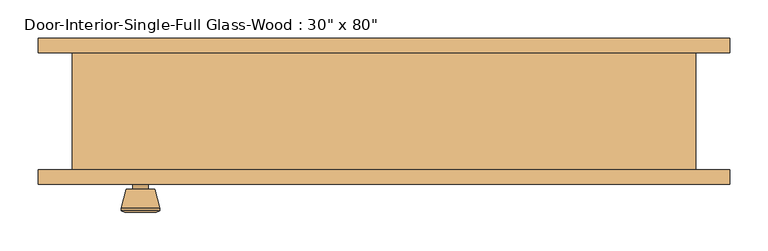
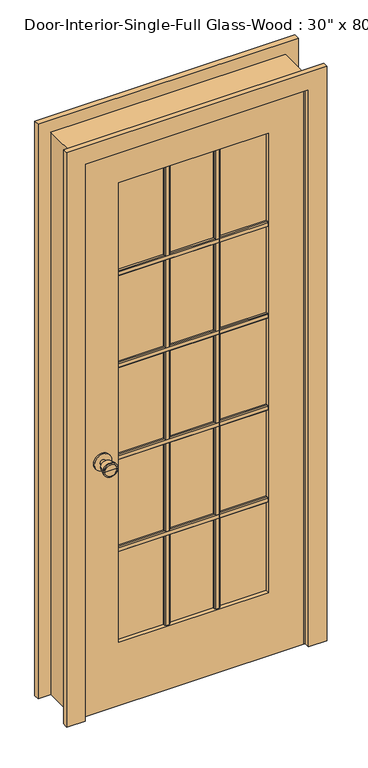
"""IFC4 building model written with IfcOpenShell, lengths in millimetres: door geometry."""

from ifc_helpers import new_model, si_unit, point, frame, frame_2d, origin, place, context, project, spatial, polyline, circle_curve, trimmed, segment, composite_curve, outline, extrude, faceted_brep, source, transform, mapped, element, save
from ifc_brep_helpers import plane_surface, cylinder_surface, revolved_surface, advanced_brep


def door_a0b5ff2a(model_context):
    return source(origin(), model_context, "Body", "SolidModel", [
        extrude(outline(polyline([(-59.055, 1586.23), (-59.055, 1567.18), (-65.405, 1567.18), (-68.58, 1570.355), (-68.58, 1583.055), (-65.405, 1586.23), (-59.055, 1586.23)])), frame((-260.35, 0.0, 0.0), z_axis=(1.0, 0.0, 0.0), x_axis=(0.0, 1.0, 0.0)), (0.0, 0.0, 1.0), 520.7),
        extrude(outline(polyline([(-59.055, 1249.9975), (-59.055, 1230.9475), (-65.405, 1230.9475), (-68.58, 1234.1225), (-68.58, 1246.8225), (-65.405, 1249.9975), (-59.055, 1249.9975)])), frame((-260.35, 0.0, 0.0), z_axis=(1.0, 0.0, 0.0), x_axis=(0.0, 1.0, 0.0)), (0.0, 0.0, 1.0), 520.7),
        extrude(outline(polyline([(-59.055, 913.765), (-59.055, 894.715), (-65.405, 894.715), (-68.58, 897.89), (-68.58, 910.59), (-65.405, 913.765), (-59.055, 913.765)])), frame((-260.35, 0.0, 0.0), z_axis=(1.0, 0.0, 0.0), x_axis=(0.0, 1.0, 0.0)), (0.0, 0.0, 1.0), 520.7),
        extrude(outline(polyline([(-59.055, 577.5325), (-59.055, 558.4825), (-65.405, 558.4825), (-68.58, 561.6575), (-68.58, 574.3575), (-65.405, 577.5325), (-59.055, 577.5325)])), frame((-260.35, 0.0, 0.0), z_axis=(1.0, 0.0, 0.0), x_axis=(0.0, 1.0, 0.0)), (0.0, 0.0, 1.0), 520.7),
        extrude(outline(polyline([(77.2583333, -59.055), (96.3083333, -59.055), (96.3083333, -65.405), (93.1333333, -68.58), (80.4333333, -68.58), (77.2583333, -65.405), (77.2583333, -59.055)])), frame((0.0, 0.0, 231.775), z_axis=(0.0, 0.0, 1.0), x_axis=(1.0, 0.0, 0.0)), (0.0, 0.0, 1.0), 1681.1625),
        extrude(outline(polyline([(-96.3083333, -59.055), (-77.2583333, -59.055), (-77.2583333, -65.405), (-80.4333333, -68.58), (-93.1333333, -68.58), (-96.3083333, -65.405), (-96.3083333, -59.055)])), frame((0.0, 0.0, 231.775), z_axis=(0.0, 0.0, 1.0), x_axis=(1.0, 0.0, 0.0)), (0.0, 0.0, 1.0), 1681.1625),
        extrude(outline(polyline([(-52.07, 1586.23), (-45.72, 1586.23), (-42.545, 1583.055), (-42.545, 1570.355), (-45.72, 1567.18), (-52.07, 1567.18), (-52.07, 1586.23)])), frame((-260.35, 0.0, 0.0), z_axis=(1.0, 0.0, 0.0), x_axis=(0.0, 1.0, 0.0)), (0.0, 0.0, 1.0), 520.7),
        extrude(outline(polyline([(-52.07, 1249.9975), (-45.72, 1249.9975), (-42.545, 1246.8225), (-42.545, 1234.1225), (-45.72, 1230.9475), (-52.07, 1230.9475), (-52.07, 1249.9975)])), frame((-260.35, 0.0, 0.0), z_axis=(1.0, 0.0, 0.0), x_axis=(0.0, 1.0, 0.0)), (0.0, 0.0, 1.0), 520.7),
        extrude(outline(polyline([(-52.07, 913.765), (-45.72, 913.765), (-42.545, 910.59), (-42.545, 897.89), (-45.72, 894.715), (-52.07, 894.715), (-52.07, 913.765)])), frame((-260.35, 0.0, 0.0), z_axis=(1.0, 0.0, 0.0), x_axis=(0.0, 1.0, 0.0)), (0.0, 0.0, 1.0), 520.7),
        extrude(outline(polyline([(-52.07, 577.5325), (-45.72, 577.5325), (-42.545, 574.3575), (-42.545, 561.6575), (-45.72, 558.4825), (-52.07, 558.4825), (-52.07, 577.5325)])), frame((-260.35, 0.0, 0.0), z_axis=(1.0, 0.0, 0.0), x_axis=(0.0, 1.0, 0.0)), (0.0, 0.0, 1.0), 520.7),
        extrude(outline(polyline([(77.2583333, -52.07), (77.2583333, -45.72), (80.4333333, -42.545), (93.1333333, -42.545), (96.3083333, -45.72), (96.3083333, -52.07), (77.2583333, -52.07)])), frame((0.0, 0.0, 231.775), z_axis=(0.0, 0.0, 1.0), x_axis=(1.0, 0.0, 0.0)), (0.0, 0.0, 1.0), 1681.1625),
        extrude(outline(polyline([(-96.3083333, -52.07), (-96.3083333, -45.72), (-93.1333333, -42.545), (-80.4333333, -42.545), (-77.2583333, -45.72), (-77.2583333, -52.07), (-96.3083333, -52.07)])), frame((0.0, 0.0, 231.775), z_axis=(0.0, 0.0, 1.0), x_axis=(1.0, 0.0, 0.0)), (0.0, 0.0, 1.0), 1681.1625),
        advanced_brep(
        [(-317.5, -32.1, 914.4), (-327.5, -32.1, 914.4), (-307.5, -32.1, 914.4), (-297.0241324, 16.9, 914.4), (-337.9758676, 16.9, 914.4), (-317.5, 16.9, 914.4), (-292.5, 15.0721319, 914.4), (-342.5, 15.0721319, 914.4), (-292.5, 11.6084537, 914.4), (-342.5, 11.6084537, 914.4), (-298.863764, -13.1, 914.4), (-336.136236, -13.1, 914.4), (-307.5, -13.1, 914.4), (-327.5, -13.1, 914.4)],
        [
            (0, 1),
            (1, 2, circle_curve(frame((-317.5, -32.1, 914.4), z_axis=(0.0, -1.0, 0.0), x_axis=(-1.0, 0.0, 0.0)), 10.0)),
            (2, 0),
            (2, 1, circle_curve(frame((-317.5, -32.1, 914.4), z_axis=(0.0, -1.0, 0.0), x_axis=(-1.0, 0.0, 0.0)), 10.0)),
            (3, 4, circle_curve(frame((-317.5, 16.9, 914.4), z_axis=(0.0, 1.0, 0.0), x_axis=(-1.0, 0.0, 0.0)), 20.4758676)),
            (4, 5),
            (5, 3),
            (4, 3, circle_curve(frame((-317.5, 16.9, 914.4), z_axis=(0.0, 1.0, 0.0), x_axis=(-1.0, 0.0, 0.0)), 20.4758676)),
            (6, 7, circle_curve(frame((-317.5, 15.0721319, 914.4), z_axis=(0.0, 1.0, 0.0), x_axis=(-1.0, 0.0, 0.0)), 25.0)),
            (7, 4),
            (3, 6),
            (7, 6, circle_curve(frame((-317.5, 15.0721319, 914.4), z_axis=(0.0, 1.0, 0.0), x_axis=(-1.0, 0.0, 0.0)), 25.0)),
            (8, 9, circle_curve(frame((-317.5, 11.6084537, 914.4), z_axis=(0.0, 1.0, 0.0), x_axis=(-1.0, 0.0, 0.0)), 25.0)),
            (9, 7),
            (6, 8),
            (9, 8, circle_curve(frame((-317.5, 11.6084537, 914.4), z_axis=(0.0, 1.0, 0.0), x_axis=(-1.0, 0.0, 0.0)), 25.0)),
            (10, 11, circle_curve(frame((-317.5, -13.1, 914.4), z_axis=(0.0, 1.0, 0.0), x_axis=(-1.0, 0.0, 0.0)), 18.636236)),
            (11, 9),
            (8, 10),
            (11, 10, circle_curve(frame((-317.5, -13.1, 914.4), z_axis=(0.0, 1.0, 0.0), x_axis=(-1.0, 0.0, 0.0)), 18.636236)),
            (12, 13, circle_curve(frame((-317.5, -13.1, 914.4), z_axis=(0.0, 1.0, 0.0), x_axis=(-1.0, 0.0, 0.0)), 10.0)),
            (13, 11),
            (10, 12),
            (13, 12, circle_curve(frame((-317.5, -13.1, 914.4), z_axis=(0.0, 1.0, 0.0), x_axis=(-1.0, 0.0, 0.0)), 10.0)),
            (1, 13),
            (12, 2),
        ],
        [
            plane_surface(frame((-317.5, -32.1, 914.4), z_axis=(0.0, -1.0, 0.0), x_axis=(-1.0, 0.0, 0.0))),
            plane_surface(frame((-317.5, 16.9, 914.4), z_axis=(0.0, 1.0, 0.0), x_axis=(-1.0, 0.0, 0.0))),
            revolved_surface(polyline([(-337.9758676, 16.9, 914.4), (-342.5, 15.0721319, 914.4)]), (-317.5, -32.1, 914.4), (0.0, -1.0, 0.0)),
            cylinder_surface(frame((-317.5, -32.1, 914.4), z_axis=(0.0, -1.0, 0.0), x_axis=(-1.0, 0.0, 0.0)), 25.0),
            revolved_surface(polyline([(-342.5, 11.6084537, 914.4), (-336.136236, -13.1, 914.4)]), (-317.5, -32.1, 914.4), (0.0, -1.0, 0.0)),
            plane_surface(frame((-317.5, -13.1, 914.4), z_axis=(0.0, -1.0, 0.0), x_axis=(-1.0, 0.0, 0.0))),
            cylinder_surface(frame((-317.5, -32.1, 914.4), z_axis=(0.0, -1.0, 0.0), x_axis=(-1.0, 0.0, 0.0)), 10.0),
        ],
        [
            (0, [[1, 2, 3]]),
            (0, [[-3, 4, -1]]),
            (1, [[5, 6, 7]]),
            (1, [[8, -7, -6]]),
            (2, [[9, 10, -5, 11]]),
            (2, [[12, -11, -8, -10]]),
            (3, [[13, 14, -9, 15]]),
            (3, [[16, -15, -12, -14]]),
            (4, [[17, 18, -13, 19]]),
            (4, [[20, -19, -16, -18]]),
            (5, [[21, 22, -17, 23]]),
            (5, [[24, -23, -20, -22]]),
            (6, [[-2, 25, -21, 26]]),
            (6, [[-4, -26, -24, -25]]),
        ],
    ),
        extrude(outline(composite_curve([segment(trimmed(circle_curve(frame_2d((914.4, -317.5)), 30.0), [point((914.4, -347.5))], [point((914.4, -287.5))], False, "CARTESIAN"), True, "CONTINUOUS"), segment(trimmed(circle_curve(frame_2d((914.4, -317.5)), 30.0), [point((914.4, -287.5))], [point((914.4, -347.5))], False, "CARTESIAN"), True, "CONTINUOUS")], self_intersect=False)), frame((0.0, -38.1, 0.0), z_axis=(0.0, 1.0, 0.0), x_axis=(0.0, 0.0, 1.0)), (0.0, 0.0, 1.0), 6.0),
        advanced_brep(
        [(-317.5, -79.025, 914.4), (-307.5, -79.025, 914.4), (-327.5, -79.025, 914.4), (-297.0241324, -128.025, 914.4), (-317.5, -128.025, 914.4), (-337.9758676, -128.025, 914.4), (-292.5, -126.1971319, 914.4), (-342.5, -126.1971319, 914.4), (-292.5, -122.7334537, 914.4), (-342.5, -122.7334537, 914.4), (-298.863764, -98.025, 914.4), (-336.136236, -98.025, 914.4), (-307.5, -98.025, 914.4), (-327.5, -98.025, 914.4)],
        [
            (0, 1),
            (1, 2, circle_curve(frame((-317.5, -79.025, 914.4), z_axis=(0.0, 1.0, 0.0), x_axis=(-1.0, 0.0, 0.0)), 10.0)),
            (2, 0),
            (2, 1, circle_curve(frame((-317.5, -79.025, 914.4), z_axis=(0.0, 1.0, 0.0), x_axis=(-1.0, 0.0, 0.0)), 10.0)),
            (3, 4),
            (4, 5),
            (5, 3, circle_curve(frame((-317.5, -128.025, 914.4), z_axis=(0.0, -1.0, 0.0), x_axis=(-1.0, 0.0, 0.0)), 20.4758676)),
            (3, 5, circle_curve(frame((-317.5, -128.025, 914.4), z_axis=(0.0, -1.0, 0.0), x_axis=(-1.0, 0.0, 0.0)), 20.4758676)),
            (6, 3),
            (5, 7),
            (7, 6, circle_curve(frame((-317.5, -126.1971319, 914.4), z_axis=(0.0, -1.0, 0.0), x_axis=(-1.0, 0.0, 0.0)), 25.0)),
            (6, 7, circle_curve(frame((-317.5, -126.1971319, 914.4), z_axis=(0.0, -1.0, 0.0), x_axis=(-1.0, 0.0, 0.0)), 25.0)),
            (8, 6),
            (7, 9),
            (9, 8, circle_curve(frame((-317.5, -122.7334537, 914.4), z_axis=(0.0, -1.0, 0.0), x_axis=(-1.0, 0.0, 0.0)), 25.0)),
            (8, 9, circle_curve(frame((-317.5, -122.7334537, 914.4), z_axis=(0.0, -1.0, 0.0), x_axis=(-1.0, 0.0, 0.0)), 25.0)),
            (10, 8),
            (9, 11),
            (11, 10, circle_curve(frame((-317.5, -98.025, 914.4), z_axis=(0.0, -1.0, 0.0), x_axis=(-1.0, 0.0, 0.0)), 18.636236)),
            (10, 11, circle_curve(frame((-317.5, -98.025, 914.4), z_axis=(0.0, -1.0, 0.0), x_axis=(-1.0, 0.0, 0.0)), 18.636236)),
            (12, 10),
            (11, 13),
            (13, 12, circle_curve(frame((-317.5, -98.025, 914.4), z_axis=(0.0, -1.0, 0.0), x_axis=(-1.0, 0.0, 0.0)), 10.0)),
            (12, 13, circle_curve(frame((-317.5, -98.025, 914.4), z_axis=(0.0, -1.0, 0.0), x_axis=(-1.0, 0.0, 0.0)), 10.0)),
            (1, 12),
            (13, 2),
        ],
        [
            plane_surface(frame((-317.5, -79.025, 914.4), z_axis=(0.0, 1.0, 0.0), x_axis=(-1.0, 0.0, 0.0))),
            plane_surface(frame((-317.5, -128.025, 914.4), z_axis=(0.0, -1.0, 0.0), x_axis=(-1.0, 0.0, 0.0))),
            revolved_surface(polyline([(-337.9758676, -128.025, 914.4), (-342.5, -126.1971319, 914.4)]), (-317.5, -79.025, 914.4), (0.0, 1.0, 0.0)),
            cylinder_surface(frame((-317.5, -79.025, 914.4), z_axis=(0.0, 1.0, 0.0), x_axis=(-1.0, 0.0, 0.0)), 25.0),
            revolved_surface(polyline([(-342.5, -122.7334537, 914.4), (-336.136236, -98.025, 914.4)]), (-317.5, -79.025, 914.4), (0.0, 1.0, 0.0)),
            plane_surface(frame((-317.5, -98.025, 914.4), z_axis=(0.0, 1.0, 0.0), x_axis=(-1.0, 0.0, 0.0))),
            cylinder_surface(frame((-317.5, -79.025, 914.4), z_axis=(0.0, 1.0, 0.0), x_axis=(-1.0, 0.0, 0.0)), 10.0),
        ],
        [
            (0, [[1, 2, 3]]),
            (0, [[-3, 4, -1]]),
            (1, [[5, 6, 7]]),
            (1, [[-6, -5, 8]]),
            (2, [[9, -7, 10, 11]]),
            (2, [[-10, -8, -9, 12]]),
            (3, [[13, -11, 14, 15]]),
            (3, [[-14, -12, -13, 16]]),
            (4, [[17, -15, 18, 19]]),
            (4, [[-18, -16, -17, 20]]),
            (5, [[21, -19, 22, 23]]),
            (5, [[-22, -20, -21, 24]]),
            (6, [[25, -23, 26, -2]]),
            (6, [[-26, -24, -25, -4]]),
        ],
    ),
        extrude(outline(composite_curve([segment(trimmed(circle_curve(frame_2d((914.4, -317.5)), 30.0), [point((914.4, -347.5))], [point((914.4, -287.5))], False, "CARTESIAN"), True, "CONTINUOUS"), segment(trimmed(circle_curve(frame_2d((914.4, -317.5)), 30.0), [point((914.4, -287.5))], [point((914.4, -347.5))], False, "CARTESIAN"), True, "CONTINUOUS")], self_intersect=False)), frame((0.0, -79.025, 0.0), z_axis=(0.0, 1.0, 0.0), x_axis=(0.0, 0.0, 1.0)), (0.0, 0.0, 1.0), 6.0),
        extrude(outline(polyline([(2032.0, -381.0), (0.0, -381.0), (0.0, 381.0), (2032.0, 381.0), (2032.0, -381.0)]), holes=[polyline([(1912.9375, -260.35), (1912.9375, 260.35), (231.775, 260.35), (231.775, -260.35), (1912.9375, -260.35)])]), frame((0.0, -73.025, 0.0), z_axis=(0.0, 1.0, 0.0), x_axis=(0.0, 0.0, 1.0)), (0.0, 0.0, 1.0), 34.925),
        faceted_brep([(406.4, -73.025, 0.0), (381.0, -73.025, 0.0), (381.0, -38.1, 0.0), (368.3, -38.1, 0.0), (368.3, -3.175, 0.0), (381.0, -3.175, 0.0), (381.0, 79.375, 0.0), (406.4, 79.375, 0.0), (406.4, 79.375, 2057.4), (406.4, -73.025, 2057.4), (381.0, 79.375, 2032.0), (-381.0, 79.375, 2032.0), (-381.0, 79.375, 0.0), (-406.4, 79.375, 0.0), (-406.4, 79.375, 2057.4), (381.0, -3.175, 2032.0), (368.3, -3.175, 2019.3), (-368.3, -3.175, 2019.3), (-368.3, -3.175, 0.0), (-381.0, -3.175, 0.0), (-381.0, -3.175, 2032.0), (368.3, -38.1, 2019.3), (381.0, -38.1, 2032.0), (-381.0, -38.1, 2032.0), (-381.0, -38.1, 0.0), (-368.3, -38.1, 0.0), (-368.3, -38.1, 2019.3), (381.0, -73.025, 2032.0), (-406.4, -73.025, 2057.4), (-406.4, -73.025, 0.0), (-381.0, -73.025, 0.0), (-381.0, -73.025, 2032.0)], [[[0, 1, 2, 3, 4, 5, 6, 7]], [[7, 8, 9, 0]], [[6, 10, 11, 12, 13, 14, 8, 7]], [[5, 15, 10, 6]], [[4, 16, 17, 18, 19, 20, 15, 5]], [[3, 21, 16, 4]], [[2, 22, 23, 24, 25, 26, 21, 3]], [[1, 27, 22, 2]], [[0, 9, 28, 29, 30, 31, 27, 1]], [[8, 14, 28, 9]], [[15, 20, 11, 10]], [[21, 26, 17, 16]], [[27, 31, 23, 22]], [[29, 13, 12, 19, 18, 25, 24, 30]], [[14, 13, 29, 28]], [[20, 19, 12, 11]], [[26, 25, 18, 17]], [[31, 30, 24, 23]]]),
        extrude(outline(polyline([(260.35, -52.07), (260.35, -59.055), (-260.35, -59.055), (-260.35, -52.07), (260.35, -52.07)])), frame((0.0, 0.0, 231.775), z_axis=(0.0, 0.0, 1.0), x_axis=(1.0, 0.0, 0.0)), (0.0, 0.0, 1.0), 1681.1625),
        extrude(outline(polyline([(0.0, 450.85), (2101.85, 450.85), (2101.85, -450.85), (0.0, -450.85), (0.0, -387.35), (2038.35, -387.35), (2038.35, 387.35), (0.0, 387.35), (0.0, 450.85)])), frame((0.0, 79.375, 0.0), z_axis=(0.0, 1.0, 0.0), x_axis=(0.0, 0.0, 1.0)), (0.0, 0.0, 1.0), 19.05),
        extrude(outline(polyline([(0.0, 450.85), (2101.85, 450.85), (2101.85, -450.85), (0.0, -450.85), (0.0, -387.35), (2038.35, -387.35), (2038.35, 387.35), (0.0, 387.35), (0.0, 450.85)])), frame((0.0, -92.075, 0.0), z_axis=(0.0, 1.0, 0.0), x_axis=(0.0, 0.0, 1.0)), (0.0, 0.0, 1.0), 19.05),
    ])


if __name__ == "__main__":
    model = new_model("IFC4")
    model_context = context("Model", 3, world=origin())
    ifc_project = project(units=[si_unit("LENGTHUNIT", "METRE", prefix="MILLI")], contexts=[model_context])
    site = spatial("IfcSite", under=ifc_project)
    building = spatial("IfcBuilding", under=site)
    placement = place(None, origin())
    door_shape = door_a0b5ff2a(model_context)
    element("IfcDoor", 1, ObjectType="Door-Interior-Single-Full Glass-Wood : 30\" x 80\"", at=placement, inside=building, context=model_context, shape_type="MappedRepresentation", body=[
        mapped(door_shape, transform((0.0, 0.0, 0.0), x_axis=(1.0, 0.0, 0.0), y_axis=(0.0, 1.0, 0.0), z_axis=(0.0, 0.0, 1.0))),
    ])
    save(model, "model.ifc")

# Revit data of these elements
# Type "Door-Interior-Single-Full Glass-Wood : 30\" x 80\""
#   Type Mark = "11"
#   Assembly Code = "C1020300"
#   Analytic Construction = "Wood frame with single clear glass"
#   Top Rail = 0' - 4 11/16"
#   Thickness = 0' - 1 3/8"
#   Thermal Resistance (R) = 1.0102 (h·ft²·°F)/BTU
#   Swing Angle [instance default] = 90.00°
#   Stiles = 0' - 4 3/4"
#   Rough Width = 2' - 8"
#   Rough Height = 6' - 9"
#   Height = 6' - 8"
#   Width = 2' - 6"
#   Heat Transfer Coefficient (U) = 0.9900 BTU/(h·ft²·°F)
#   Bottom Rail = 0' - 9 1/8"
#   Show Grill [instance default] = yes
#   Trim Material = Cherry
#   Panel Material = Cherry
#   Frame Material = Cherry
#   Door Handle Material = Aluminum
#   Visual Light Transmittance = 0
#   Solar Heat Gain Coefficient = 0
#   Wall Closure = (empty or 0)
#   Function = (empty or 0)
# Element 1 (IfcDoor, "Door-Interior-Single-Full Glass-Wood : 30\" x 80\"")
#   Materials on its faces: "Cherry", "Aluminum", "Glass"
# Materials
#   "Cherry": class "Wood", colour RGB 226 177 128, transparency 0, Description = "Prunus Serotina", Cost = 0
#   "Aluminum": class "Metal", colour RGB 247 247 247, transparency 0, Description = "Aluminum 6061", Cost = 0
#   "Glass": class "Glass", colour RGB 0 128 192, transparency 0.75, Description = "Soda Lime Glass", Cost = 0
